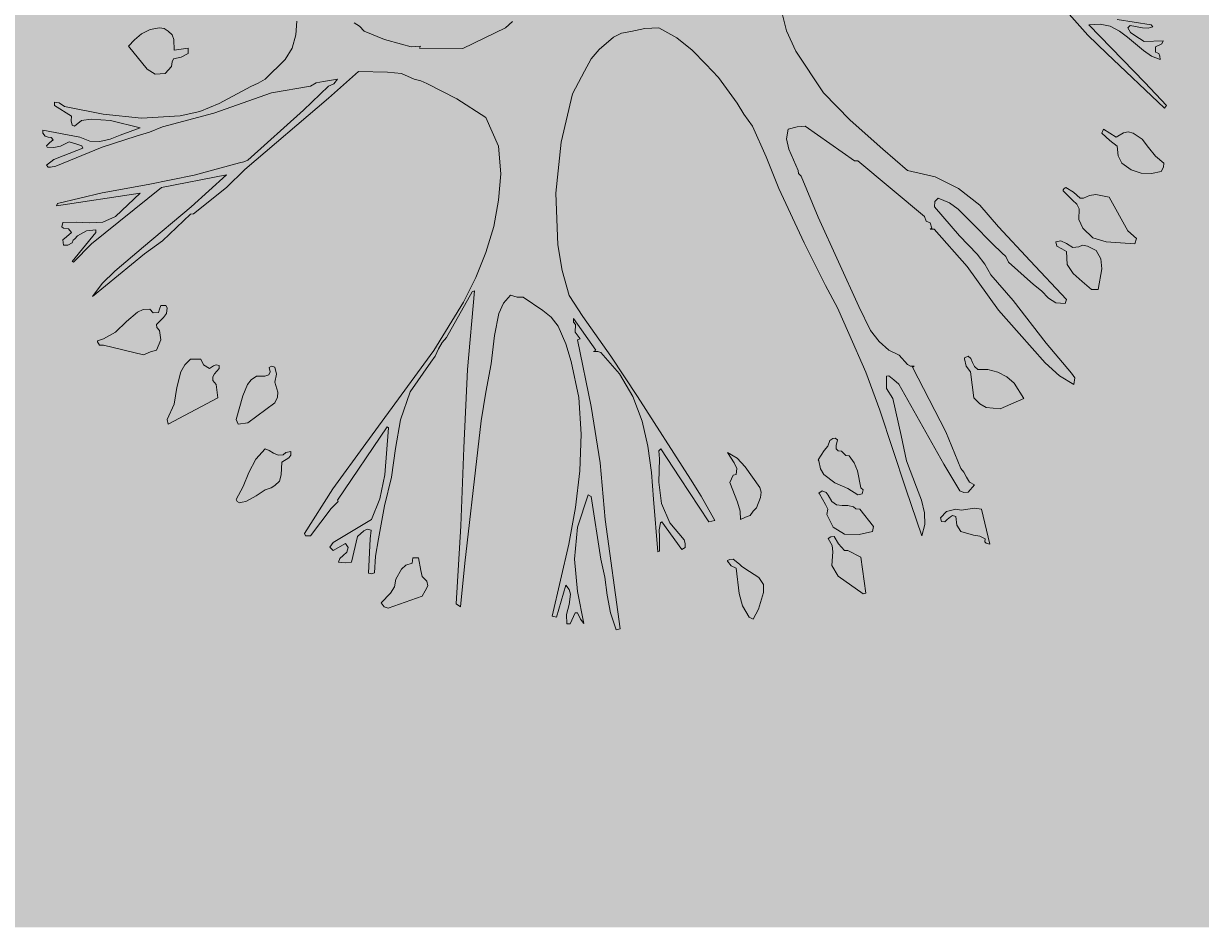
# Model space of a CAD drawing. Units: inches. Extents: x 84 to 1044, y -280 to 906.
# Tile 54 of 105: x 389 to 412, y 709 to 726. Entities that reach past the tile are written whole.
import ezdxf

# ---------------------------------------------------------------- set-up
doc = ezdxf.new("R2010")
doc.units = ezdxf.units.IN
doc.layers.add('A-ANNO-DIMS', color=2, linetype='Continuous', lineweight=18)
doc.layers.add('L-PLNT', color=114, linetype='Continuous', lineweight=15)
doc.layers.add('L-PLNT-PATT', color=9, linetype='Continuous', lineweight=9, true_color=0xafd9aa)
doc.styles.get("Standard").update_dxf_attribs({"font": 'arial.ttf'})
doc.dimstyles.get("Standard").update_dxf_attribs({"dimtxt": 0.18, "dimasz": 0.18, "dimexe": 0.18, "dimexo": 0.0625, "dimgap": 0.09, "dimtad": 0, "dimtih": 1, "dimtoh": 1, "dimdec": 4, "dimzin": 0, "dimdsep": 46, "dimtxsty": 'Standard', "dimcen": 0.09, "dimadec": 0, "dimazin": 0, "dimtfac": 1, "dimtdec": 4, "dimtofl": 0, "dimtmove": 0, "dimatfit": 3, "dimfxl": 1, "dimtolj": 1, "dimtzin": 0, "dimarcsym": 0})

# ---------------------------------------------------------------- blocks, each defined once
blk = doc.blocks.new('A$C37E508DF')
for p, q in [((0.9287, 0.7825), (0.936, 0.7542)), ((1.3151, 0.7487), (1.2919, 0.7752)), ((0.1244, 0.7504), (0.1351, 0.7559)), ((0.1351, 0.7559), (0.1471, 0.7577)), ((0.1471, 0.7577), (0.1527, 0.7568)), ((0.1527, 0.7568), (0.1578, 0.7538)), ((0.3186, 0.7491), (0.3199, 0.7662)), ((0.3919, 0.7641), (0.3988, 0.7598)), ((0.3988, 0.7598), (0.4043, 0.7538)), ((0.5287, 0.7319), (0.5823, 0.7577)), ((0.5823, 0.7577), (0.5913, 0.7658)), ((0.7577, 0.7568), (0.7401, 0.7534)), ((0.7752, 0.7577), (0.7577, 0.7568)), ((0.798, 0.7452), (0.7752, 0.7577)), ((1.3309, 0.7624), (1.3164, 0.7615)), ((1.3164, 0.7615), (1.3871, 0.6891)), ((1.3434, 0.7598), (1.3309, 0.7624)), ((1.355, 0.7538), (1.3434, 0.7598)), ((1.352, 0.7684), (1.3948, 0.7615)), ((1.3687, 0.7607), (1.3657, 0.7577)), ((1.3657, 0.7577), (1.3691, 0.7521)), ((1.3841, 0.7577), (1.3687, 0.7607)), ((1.3914, 0.7572), (1.3841, 0.7577)), ((1.397, 0.759), (1.3914, 0.7572)), ((1.3948, 0.7615), (1.397, 0.759)), ((0.1081, 0.7349), (0.1153, 0.7427)), ((0.1153, 0.7427), (0.1244, 0.7504)), ((0.1578, 0.7538), (0.1629, 0.7491)), ((0.1629, 0.7491), (0.1651, 0.7431)), ((0.1651, 0.7431), (0.1655, 0.7298)), ((0.3139, 0.7324), (0.3186, 0.7491)), ((0.4043, 0.7538), (0.4301, 0.7431)), ((0.4301, 0.7431), (0.4515, 0.7371)), ((0.7182, 0.7461), (0.7002, 0.7307)), ((0.7285, 0.7512), (0.7182, 0.7461)), ((0.7401, 0.7534), (0.7285, 0.7512)), ((0.8173, 0.7298), (0.798, 0.7452)), ((0.936, 0.7542), (0.9476, 0.7285)), ((1.3391, 0.7255), (1.3151, 0.7487)), ((1.3653, 0.7461), (1.355, 0.7538)), ((1.3854, 0.7294), (1.3653, 0.7461)), ((1.3691, 0.7521), (1.3743, 0.7482)), ((1.3743, 0.7482), (1.3863, 0.7405)), ((1.3863, 0.7405), (1.4099, 0.7414)), ((1.4099, 0.7414), (1.4086, 0.7375)), ((0.1312, 0.7058), (0.1081, 0.7349)), ((0.1655, 0.7298), (0.1831, 0.7324)), ((0.1831, 0.7324), (0.1831, 0.7255)), ((0.3049, 0.7178), (0.3139, 0.7324)), ((0.4515, 0.7371), (0.4635, 0.7341)), ((0.4635, 0.7341), (0.4755, 0.7349)), ((0.4755, 0.7349), (0.4742, 0.7324)), ((0.4742, 0.7324), (0.5287, 0.7319)), ((0.7002, 0.7307), (0.6903, 0.7186)), ((0.8344, 0.7122), (0.8173, 0.7298)), ((0.9476, 0.7285), (0.9828, 0.6762)), ((1.3953, 0.7221), (1.3854, 0.7294)), ((1.4086, 0.7375), (1.4004, 0.7337)), ((1.4004, 0.7337), (1.4004, 0.7272)), ((1.4004, 0.7272), (1.4047, 0.7255)), ((0.1629, 0.7152), (0.1621, 0.7092)), ((0.1646, 0.7186), (0.1629, 0.7152)), ((0.1741, 0.7208), (0.1646, 0.7186)), ((0.1831, 0.7255), (0.1741, 0.7208)), ((0.28, 0.6933), (0.3049, 0.7178)), ((0.6903, 0.7186), (0.6818, 0.7032)), ((0.8503, 0.6951), (0.8344, 0.7122)), ((1.4116, 0.6569), (1.3391, 0.7255)), ((1.4064, 0.7178), (1.3953, 0.7221)), ((1.4047, 0.7255), (1.406, 0.7221)), ((1.406, 0.7221), (1.4064, 0.7178)), ((0.1415, 0.6994), (0.1312, 0.7058)), ((0.1539, 0.7002), (0.1415, 0.6994)), ((0.1621, 0.7092), (0.1539, 0.7002)), ((0.3975, 0.7028), (0.3598, 0.6693)), ((0.4339, 0.7019), (0.3975, 0.7028)), ((0.4515, 0.7002), (0.4339, 0.7019)), ((0.4674, 0.6933), (0.4515, 0.7002)), ((0.6818, 0.7032), (0.6667, 0.6749)), ((0.2221, 0.6625), (0.262, 0.6839)), ((0.262, 0.6839), (0.271, 0.6882)), ((0.271, 0.6882), (0.28, 0.6933)), ((0.337, 0.6843), (0.2877, 0.6762)), ((0.328, 0.6543), (0.3598, 0.6843)), ((0.3443, 0.6886), (0.337, 0.6843)), ((0.3533, 0.6903), (0.3443, 0.6886)), ((0.3709, 0.6933), (0.3533, 0.6903)), ((0.3598, 0.6843), (0.3662, 0.6873)), ((0.3662, 0.6873), (0.3709, 0.6933)), ((0.476, 0.6912), (0.4674, 0.6933)), ((0.4832, 0.6878), (0.476, 0.6912)), ((0.521, 0.6685), (0.4832, 0.6878)), ((0.8739, 0.6629), (0.8503, 0.6951)), ((1.3871, 0.6891), (1.4141, 0.6599)), ((0.2877, 0.6762), (0.2152, 0.6505)), ((0.3598, 0.6693), (0.2543, 0.5797)), ((0.5578, 0.6449), (0.521, 0.6685)), ((0.6667, 0.6749), (0.6526, 0.614)), ((0.9828, 0.6762), (1.0162, 0.6415)), ((0.0146, 0.6599), (0.0146, 0.6642)), ((0.0146, 0.6642), (0.0206, 0.6633)), ((0.036, 0.6466), (0.0146, 0.6599)), ((0.0206, 0.6633), (0.0274, 0.6586)), ((0.0274, 0.6586), (0.0759, 0.6492)), ((0.1728, 0.647), (0.1977, 0.6526)), ((0.1977, 0.6526), (0.2221, 0.6625)), ((0.2581, 0.5913), (0.328, 0.6543)), ((0.8824, 0.6492), (0.8739, 0.6629)), ((1.4141, 0.6599), (1.4116, 0.6569)), ((0.0356, 0.6406), (0.036, 0.6466)), ((0.0369, 0.6355), (0.0356, 0.6406)), ((0.0489, 0.641), (0.0399, 0.6342)), ((0.0609, 0.6428), (0.0489, 0.641)), ((0.0853, 0.641), (0.0609, 0.6428)), ((0.0759, 0.6492), (0.1244, 0.644)), ((0.1226, 0.632), (0.0853, 0.641)), ((0.1244, 0.644), (0.1728, 0.647)), ((0.2152, 0.6505), (0.1509, 0.6333)), ((0.5737, 0.6089), (0.5578, 0.6449)), ((0.8932, 0.6342), (0.8824, 0.6492)), ((1.0162, 0.6415), (1.0574, 0.605)), ((0, 0.629), (0.0467, 0.62)), ((0, 0.6252), (0, 0.629)), ((0.003, 0.6213), (0, 0.6252)), ((0.0399, 0.6342), (0.0369, 0.6355)), ((0.0849, 0.6175), (0.0973, 0.6226)), ((0.0973, 0.6226), (0.1226, 0.632)), ((0.1342, 0.6265), (0.1175, 0.6213)), ((0.1509, 0.6333), (0.1342, 0.6265)), ((0.9103, 0.5956), (0.8932, 0.6342)), ((0.9382, 0.6303), (0.936, 0.6179)), ((0.9493, 0.6333), (0.9382, 0.6303)), ((0.9596, 0.6342), (0.9493, 0.6333)), ((1.0218, 0.5904), (0.9596, 0.6342)), ((1.3327, 0.6252), (1.3348, 0.6303)), ((1.343, 0.6162), (1.3327, 0.6252)), ((1.3348, 0.6303), (1.3511, 0.62)), ((1.3511, 0.62), (1.3601, 0.6256)), ((1.3601, 0.6256), (1.3661, 0.6269)), ((1.3661, 0.6269), (1.3725, 0.6252)), ((1.3725, 0.6252), (1.3837, 0.6175)), ((0.0069, 0.6204), (0.003, 0.6213)), ((0.0047, 0.6093), (0.0086, 0.6132)), ((0.0056, 0.6076), (0.0047, 0.6093)), ((0.0141, 0.6072), (0.0056, 0.6076)), ((0.0107, 0.6196), (0.0069, 0.6204)), ((0.0086, 0.6132), (0.0133, 0.617)), ((0.0133, 0.617), (0.0107, 0.6196)), ((0.0223, 0.6089), (0.0141, 0.6072)), ((0.0746, 0.6076), (0.0163, 0.5836)), ((0.0334, 0.6145), (0.0223, 0.6089)), ((0.0416, 0.6119), (0.0334, 0.6145)), ((0.0493, 0.6093), (0.0416, 0.6119)), ((0.0467, 0.62), (0.0592, 0.6153)), ((0.0506, 0.6063), (0.0493, 0.6093)), ((0.0592, 0.6153), (0.072, 0.6149)), ((0.072, 0.6149), (0.0849, 0.6175)), ((0.1175, 0.6213), (0.0746, 0.6076)), ((0.5763, 0.5741), (0.5737, 0.6089)), ((0.6526, 0.614), (0.6457, 0.5497)), ((0.936, 0.6179), (0.939, 0.605)), ((1.352, 0.6089), (1.343, 0.6162)), ((1.3533, 0.5969), (1.352, 0.6089)), ((1.3837, 0.6175), (1.3918, 0.6072)), ((0.0141, 0.5921), (0.0257, 0.5969)), ((0.0257, 0.5969), (0.0506, 0.6063)), ((0.9262, 0.5557), (0.9103, 0.5956)), ((0.939, 0.605), (0.9506, 0.5784)), ((1.0574, 0.605), (1.0883, 0.5784)), ((1.358, 0.5874), (1.3533, 0.5969)), ((1.3918, 0.6072), (1.4004, 0.5964)), ((1.4004, 0.5964), (1.4111, 0.5874)), ((0.0047, 0.5849), (0.0141, 0.5921)), ((0.0069, 0.5823), (0.0047, 0.5849)), ((0.0099, 0.5823), (0.0069, 0.5823)), ((0.0163, 0.5836), (0.0099, 0.5823)), ((0.1904, 0.5724), (0.2474, 0.5879)), ((0.2543, 0.5797), (0.2311, 0.557)), ((0.2474, 0.5879), (0.253, 0.5892)), ((0.253, 0.5892), (0.2581, 0.5913)), ((0.9506, 0.5784), (0.951, 0.5746)), ((1.0256, 0.5904), (1.0218, 0.5904)), ((1.1097, 0.5205), (1.0256, 0.5904)), ((1.0883, 0.5784), (1.123, 0.5703)), ((1.37, 0.5789), (1.358, 0.5874)), ((1.3824, 0.575), (1.37, 0.5789)), ((1.4103, 0.5823), (1.4077, 0.5771)), ((1.4111, 0.5874), (1.4103, 0.5823)), ((0.1325, 0.5608), (0.1904, 0.5724)), ((0.2311, 0.5729), (0.1496, 0.557)), ((0.1869, 0.5325), (0.2311, 0.5729)), ((0.5737, 0.5407), (0.5763, 0.5741)), ((0.951, 0.5746), (0.9545, 0.5711)), ((0.9545, 0.5711), (0.9759, 0.5193)), ((1.123, 0.5703), (1.1526, 0.5557)), ((1.3953, 0.5746), (1.3824, 0.575)), ((1.4077, 0.5771), (1.3953, 0.5746)), ((0.1226, 0.5497), (0.0171, 0.5338)), ((0.0184, 0.5368), (0.0746, 0.5501)), ((0.1496, 0.557), (0.0613, 0.4858)), ((0.0746, 0.5501), (0.1325, 0.5608)), ((0.0917, 0.5205), (0.1226, 0.5497)), ((0.2311, 0.557), (0.1899, 0.5235)), ((0.6457, 0.5497), (0.6483, 0.4845)), ((0.9583, 0.4871), (0.9262, 0.5557)), ((1.1526, 0.5557), (1.1792, 0.5347)), ((1.2842, 0.554), (1.2855, 0.5557)), ((1.2842, 0.5527), (1.2842, 0.554)), ((1.2958, 0.5407), (1.2842, 0.5527)), ((1.2855, 0.5557), (1.2876, 0.557)), ((1.2876, 0.557), (1.2971, 0.551)), ((1.2971, 0.551), (1.3057, 0.5433)), ((0.0171, 0.5338), (0.0184, 0.5368)), ((0.5677, 0.5077), (0.5737, 0.5407)), ((1.1226, 0.5394), (1.1221, 0.5325)), ((1.1268, 0.5433), (1.1226, 0.5394)), ((1.141, 0.5377), (1.1268, 0.5433)), ((1.1521, 0.5296), (1.141, 0.5377)), ((1.1792, 0.5347), (1.2027, 0.5072)), ((1.3014, 0.536), (1.2958, 0.5407)), ((1.3044, 0.53), (1.3014, 0.536)), ((1.3057, 0.5433), (1.3099, 0.5433)), ((1.3099, 0.5433), (1.3172, 0.5467)), ((1.3172, 0.5467), (1.3254, 0.548)), ((1.3254, 0.548), (1.3421, 0.5446)), ((1.3421, 0.5446), (1.3657, 0.5021)), ((0.0755, 0.5133), (0.0917, 0.5205)), ((0.1269, 0.482), (0.1869, 0.5325)), ((0.1861, 0.5231), (0.1509, 0.4897)), ((0.1899, 0.5235), (0.1861, 0.5231)), ((0.9759, 0.5193), (1.0269, 0.4069)), ((1.1118, 0.5145), (1.1097, 0.5205)), ((1.1221, 0.5325), (1.1539, 0.4961)), ((1.1706, 0.5111), (1.1521, 0.5296)), ((1.3039, 0.5167), (1.3044, 0.53)), ((0.024, 0.5072), (0.0253, 0.5128)), ((0.0262, 0.5055), (0.024, 0.5072)), ((0.0253, 0.5128), (0.042, 0.5133)), ((0.0326, 0.5047), (0.0262, 0.5055)), ((0.036, 0.5004), (0.0326, 0.5047)), ((0.042, 0.5133), (0.0587, 0.5124)), ((0.0587, 0.5124), (0.0755, 0.5133)), ((0.5578, 0.4751), (0.5677, 0.5077)), ((1.117, 0.5124), (1.1118, 0.5145)), ((1.1191, 0.5055), (1.117, 0.5124)), ((1.117, 0.5042), (1.1191, 0.5055)), ((1.1217, 0.5042), (1.117, 0.5042)), ((1.1633, 0.4575), (1.1217, 0.5042)), ((1.1955, 0.4858), (1.1706, 0.5111)), ((1.2027, 0.5072), (1.2426, 0.4644)), ((1.3091, 0.5055), (1.3039, 0.5167)), ((1.3215, 0.4935), (1.3091, 0.5055)), ((0.0253, 0.491), (0.03, 0.4948)), ((0.0262, 0.4841), (0.0253, 0.491)), ((0.03, 0.4948), (0.036, 0.5004)), ((0.0369, 0.4639), (0.0669, 0.5004)), ((0.0382, 0.4905), (0.0369, 0.4871)), ((0.0403, 0.4922), (0.0382, 0.4905)), ((0.0437, 0.4961), (0.0403, 0.4922)), ((0.0549, 0.5021), (0.0437, 0.4961)), ((0.0669, 0.5034), (0.0549, 0.5021)), ((0.0669, 0.5004), (0.0669, 0.5034)), ((0.1509, 0.4897), (0.1282, 0.4734)), ((1.1539, 0.4961), (1.1762, 0.4729)), ((1.2748, 0.4884), (1.2812, 0.4897)), ((1.2812, 0.4897), (1.2885, 0.4862)), ((1.3382, 0.4884), (1.3215, 0.4935)), ((1.3657, 0.5021), (1.3764, 0.4927)), ((1.3764, 0.4927), (1.3743, 0.4858)), ((0.0317, 0.4841), (0.0262, 0.4841)), ((0.0369, 0.4871), (0.0317, 0.4841)), ((0.0613, 0.4858), (0.0386, 0.4627)), ((0.0905, 0.4515), (0.1269, 0.482)), ((0.545, 0.4434), (0.5578, 0.4751)), ((0.6483, 0.4845), (0.6539, 0.4524)), ((0.9853, 0.4335), (0.9583, 0.4871)), ((1.207, 0.4747), (1.1955, 0.4858)), ((1.2122, 0.47), (1.207, 0.4747)), ((1.2761, 0.4832), (1.2748, 0.4884)), ((1.2825, 0.4798), (1.2761, 0.4832)), ((1.2885, 0.4764), (1.2825, 0.4798)), ((1.2885, 0.4862), (1.2962, 0.4815)), ((1.2894, 0.4601), (1.2885, 0.4764)), ((1.2962, 0.4815), (1.3039, 0.482)), ((1.3039, 0.482), (1.3087, 0.4841)), ((1.3087, 0.4841), (1.3147, 0.4832)), ((1.3147, 0.4832), (1.3258, 0.4777)), ((1.3258, 0.4777), (1.3318, 0.4669)), ((1.3743, 0.4858), (1.3382, 0.4884)), ((0.0386, 0.4627), (0.0369, 0.4639)), ((0.1282, 0.4734), (0.0626, 0.4198)), ((1.1762, 0.4729), (1.1856, 0.4605)), ((1.1856, 0.4605), (1.1933, 0.4468)), ((1.2156, 0.4627), (1.2122, 0.47)), ((1.2469, 0.4348), (1.2156, 0.4627)), ((1.2426, 0.4644), (1.2885, 0.4159)), ((1.2967, 0.4485), (1.2894, 0.4601)), ((1.3318, 0.4669), (1.3331, 0.4545)), ((0.0746, 0.4361), (0.0905, 0.4515)), ((0.6539, 0.4524), (0.6625, 0.4211)), ((1.2027, 0.4026), (1.1633, 0.4575)), ((1.1933, 0.4468), (1.2212, 0.4146)), ((1.3082, 0.4386), (1.2967, 0.4485)), ((1.3331, 0.4545), (1.3284, 0.4284)), ((0.0626, 0.4198), (0.0746, 0.4361)), ((0.5295, 0.4125), (0.545, 0.4434)), ((1.0003, 0.4052), (0.9853, 0.4335)), ((1.2568, 0.4266), (1.2469, 0.4348)), ((1.3198, 0.4284), (1.3082, 0.4386)), ((0.5403, 0.4254), (0.5081, 0.3679)), ((0.5347, 0.3276), (0.5433, 0.4266)), ((0.5433, 0.4266), (0.5403, 0.4254)), ((0.5887, 0.4215), (0.5797, 0.4112)), ((0.5969, 0.4189), (0.5887, 0.4215)), ((0.6046, 0.4189), (0.5969, 0.4189)), ((0.6295, 0.4022), (0.6046, 0.4189)), ((0.6625, 0.4211), (0.6796, 0.3945)), ((1.2658, 0.4176), (1.2568, 0.4266)), ((1.2752, 0.4116), (1.2658, 0.4176)), ((1.2885, 0.4159), (1.2868, 0.4108)), ((1.3284, 0.4284), (1.3198, 0.4284)), ((0.1055, 0.388), (0.1192, 0.4001)), ((0.1192, 0.4001), (0.1265, 0.4031)), ((0.1265, 0.4031), (0.1346, 0.4039)), ((0.1346, 0.4039), (0.1389, 0.3992)), ((0.1458, 0.3996), (0.1471, 0.4035)), ((0.1471, 0.4035), (0.1484, 0.4082)), ((0.1484, 0.4082), (0.1548, 0.4082)), ((0.1548, 0.4082), (0.1565, 0.4052)), ((0.1565, 0.4052), (0.1556, 0.3983)), ((0.4922, 0.3516), (0.5295, 0.4125)), ((0.5797, 0.4112), (0.5741, 0.3983)), ((0.6397, 0.3936), (0.6295, 0.4022)), ((1.0145, 0.373), (1.0003, 0.4052)), ((1.0269, 0.4069), (1.0419, 0.3769)), ((1.2289, 0.373), (1.2027, 0.4026)), ((1.2212, 0.4146), (1.2628, 0.361)), ((1.2868, 0.4108), (1.2752, 0.4116)), ((0.0917, 0.3748), (0.1055, 0.388)), ((0.1389, 0.3992), (0.1458, 0.3996)), ((0.1518, 0.3932), (0.1432, 0.3842)), ((0.1556, 0.3983), (0.1518, 0.3932)), ((0.5741, 0.3983), (0.5686, 0.3705)), ((0.6487, 0.3825), (0.6397, 0.3936)), ((0.6959, 0.352), (0.668, 0.3919)), ((0.668, 0.3919), (0.668, 0.3872)), ((0.668, 0.3872), (0.6706, 0.3842)), ((0.6796, 0.3945), (0.7148, 0.3447)), ((0.0763, 0.3662), (0.0917, 0.3748)), ((0.1432, 0.3842), (0.1436, 0.3808)), ((0.1436, 0.3808), (0.1471, 0.3769)), ((0.1471, 0.3769), (0.1484, 0.3649)), ((0.5686, 0.3705), (0.5643, 0.3349)), ((0.6582, 0.3602), (0.6487, 0.3825)), ((0.6706, 0.3842), (0.6702, 0.3748)), ((0.6702, 0.3748), (0.6762, 0.3662)), ((1.0359, 0.3246), (1.0145, 0.373)), ((1.0419, 0.3769), (1.0527, 0.3632)), ((1.2615, 0.3362), (1.2289, 0.373)), ((0.069, 0.364), (0.0763, 0.3662)), ((0.069, 0.3627), (0.069, 0.364)), ((0.0716, 0.3585), (0.069, 0.3627)), ((0.0763, 0.3585), (0.0716, 0.3585)), ((0.1269, 0.3464), (0.0763, 0.3585)), ((0.1484, 0.3649), (0.1432, 0.352)), ((0.5025, 0.3619), (0.4982, 0.3537)), ((0.5081, 0.3679), (0.5025, 0.3619)), ((0.665, 0.3379), (0.6582, 0.3602)), ((0.6762, 0.3662), (0.6732, 0.3653)), ((0.6732, 0.3653), (0.6903, 0.2813)), ((1.0527, 0.3632), (1.0647, 0.352)), ((1.2628, 0.361), (1.2949, 0.3233)), ((0.1355, 0.3499), (0.1269, 0.3464)), ((0.1432, 0.352), (0.1355, 0.3499)), ((0.1788, 0.3336), (0.1861, 0.3409)), ((0.1861, 0.3409), (0.199, 0.3409)), ((0.199, 0.3409), (0.2024, 0.3336)), ((0.4065, 0.2345), (0.4922, 0.3516)), ((0.4939, 0.3447), (0.4884, 0.337)), ((0.4982, 0.3537), (0.4939, 0.3447)), ((0.6933, 0.3503), (0.6959, 0.352)), ((0.6985, 0.3503), (0.6933, 0.3503)), ((0.7023, 0.349), (0.6985, 0.3503)), ((0.7259, 0.3224), (0.7023, 0.349)), ((0.7148, 0.3447), (0.7487, 0.2937)), ((1.0647, 0.352), (1.078, 0.346)), ((1.078, 0.346), (1.0883, 0.334)), ((1.1599, 0.3426), (1.1646, 0.3447)), ((1.1599, 0.3413), (1.1599, 0.3426)), ((1.162, 0.3319), (1.1599, 0.3413)), ((1.1646, 0.3447), (1.168, 0.3417)), ((1.168, 0.3417), (1.1702, 0.3366)), ((0.1737, 0.325), (0.1788, 0.3336)), ((0.2024, 0.3336), (0.2097, 0.3289)), ((0.2097, 0.3289), (0.2148, 0.3323)), ((0.2148, 0.3323), (0.2182, 0.3336)), ((0.2221, 0.3289), (0.2161, 0.3224)), ((0.2182, 0.3336), (0.2221, 0.3327)), ((0.2221, 0.3327), (0.2221, 0.3289)), ((0.2851, 0.3302), (0.2877, 0.3319)), ((0.2864, 0.325), (0.2851, 0.3302)), ((0.2877, 0.3319), (0.292, 0.3306)), ((0.292, 0.3306), (0.2941, 0.322)), ((0.4884, 0.337), (0.4622, 0.2997)), ((0.53, 0.229), (0.5347, 0.3276)), ((0.5643, 0.3349), (0.5578, 0.2993)), ((0.6745, 0.2924), (0.665, 0.3379)), ((1.0883, 0.334), (1.0921, 0.3319)), ((1.0921, 0.3319), (1.0968, 0.3319)), ((1.0968, 0.3319), (1.0947, 0.3306)), ((1.0947, 0.3306), (1.1367, 0.2491)), ((1.1676, 0.325), (1.162, 0.3319)), ((1.1702, 0.3366), (1.1727, 0.3314)), ((1.1727, 0.3314), (1.177, 0.3276)), ((1.177, 0.3276), (1.1895, 0.3276)), ((1.1895, 0.3276), (1.2019, 0.3246)), ((1.2795, 0.3199), (1.2615, 0.3362)), ((0.1689, 0.3053), (0.1737, 0.325)), ((0.2161, 0.3224), (0.214, 0.3186)), ((0.214, 0.3186), (0.214, 0.3139)), ((0.214, 0.3139), (0.2182, 0.3087)), ((0.2577, 0.3087), (0.2624, 0.3147)), ((0.2624, 0.3147), (0.2689, 0.3194)), ((0.2689, 0.3194), (0.2796, 0.3194)), ((0.2796, 0.3194), (0.2847, 0.3211)), ((0.2847, 0.3211), (0.2864, 0.325)), ((0.2941, 0.322), (0.292, 0.3117)), ((0.292, 0.3117), (0.2959, 0.2993)), ((0.7427, 0.2937), (0.7259, 0.3224)), ((1.0535, 0.2766), (1.0359, 0.3246)), ((1.0647, 0.3199), (1.0617, 0.3194)), ((1.0617, 0.3194), (1.0617, 0.304)), ((1.0711, 0.3147), (1.0647, 0.3199)), ((1.0775, 0.3092), (1.0711, 0.3147)), ((1.1719, 0.292), (1.1676, 0.325)), ((1.2019, 0.3246), (1.2135, 0.3186)), ((1.2135, 0.3186), (1.2225, 0.3104)), ((1.2975, 0.3087), (1.2795, 0.3199)), ((1.2949, 0.3233), (1.2988, 0.3173)), ((1.2988, 0.3173), (1.2975, 0.3087)), ((0.1655, 0.2843), (0.1689, 0.3053)), ((0.2182, 0.3087), (0.2204, 0.292)), ((0.2517, 0.2946), (0.2577, 0.3087)), ((0.2959, 0.2993), (0.2954, 0.2928)), ((0.4622, 0.2997), (0.4502, 0.2645)), ((0.5578, 0.2993), (0.5518, 0.2633)), ((1.0617, 0.304), (1.0698, 0.2911)), ((1.1341, 0.2084), (1.0775, 0.3092)), ((1.2225, 0.3104), (1.2349, 0.2911)), ((0.1565, 0.265), (0.1655, 0.2843)), ((0.2204, 0.292), (0.1578, 0.259)), ((0.2436, 0.265), (0.2517, 0.2946)), ((0.292, 0.286), (0.2581, 0.2607)), ((0.2954, 0.2928), (0.292, 0.286)), ((0.6775, 0.2465), (0.6745, 0.2924)), ((0.7542, 0.2628), (0.7427, 0.2937)), ((0.7487, 0.2937), (0.8151, 0.1899)), ((1.0698, 0.2911), (1.0805, 0.2448)), ((1.1792, 0.2847), (1.1719, 0.292)), ((1.1873, 0.28), (1.1792, 0.2847)), ((1.2349, 0.2911), (1.2049, 0.2783)), ((0.6903, 0.2813), (0.7015, 0.2101)), ((1.0861, 0.1775), (1.0535, 0.2766)), ((1.2049, 0.2783), (1.1873, 0.28)), ((0.1578, 0.259), (0.1565, 0.265)), ((0.2461, 0.259), (0.2436, 0.265)), ((0.2581, 0.2607), (0.2461, 0.259)), ((0.4335, 0.2556), (0.3709, 0.1634)), ((0.4305, 0.1951), (0.4352, 0.2543)), ((0.4352, 0.2543), (0.4335, 0.2556)), ((0.4502, 0.2645), (0.4438, 0.2285)), ((0.5518, 0.2633), (0.5475, 0.2268)), ((0.7615, 0.2311), (0.7542, 0.2628)), ((0.6758, 0.2002), (0.6775, 0.2465)), ((0.9879, 0.2311), (0.9905, 0.2384)), ((0.9905, 0.2384), (0.9943, 0.241)), ((0.9943, 0.241), (0.9973, 0.2414)), ((0.9973, 0.2414), (1.0003, 0.2393)), ((1.0003, 0.2393), (0.9986, 0.232)), ((1.0805, 0.2448), (1.087, 0.2127)), ((1.1367, 0.2491), (1.1556, 0.2032)), ((0.268, 0.2148), (0.28, 0.2277)), ((0.28, 0.2277), (0.2851, 0.226)), ((0.2851, 0.226), (0.2903, 0.2225)), ((0.2903, 0.2225), (0.2963, 0.22)), ((0.3027, 0.2204), (0.3061, 0.2234)), ((0.3061, 0.2234), (0.3122, 0.2247)), ((0.3122, 0.2247), (0.3122, 0.22)), ((0.3649, 0.1775), (0.4065, 0.2345)), ((0.4438, 0.2285), (0.4391, 0.1921)), ((0.5261, 0.1308), (0.53, 0.229)), ((0.5475, 0.2268), (0.5313, 0.084)), ((0.7662, 0.1981), (0.7615, 0.2311)), ((0.7778, 0.2277), (0.7752, 0.2255)), ((0.7752, 0.2255), (0.7761, 0.2152)), ((0.8018, 0.1912), (0.7778, 0.2277)), ((0.8619, 0.2234), (0.8739, 0.2161)), ((0.87, 0.2101), (0.8619, 0.2234)), ((0.9759, 0.214), (0.9836, 0.226)), ((0.9836, 0.226), (0.9879, 0.2311)), ((0.9986, 0.232), (0.9986, 0.2281)), ((0.9986, 0.2281), (1.0012, 0.2255)), ((1.0012, 0.2255), (1.0051, 0.2251)), ((1.0051, 0.2251), (1.0076, 0.2225)), ((1.0076, 0.2225), (1.0106, 0.2195)), ((0.2594, 0.1981), (0.268, 0.2148)), ((0.2963, 0.22), (0.3027, 0.2204)), ((0.301, 0.211), (0.3002, 0.1951)), ((0.3096, 0.2165), (0.301, 0.211)), ((0.3122, 0.22), (0.3096, 0.2165)), ((0.7015, 0.2101), (0.7079, 0.1389)), ((0.7761, 0.2152), (0.7752, 0.1861)), ((0.8734, 0.2032), (0.87, 0.2101)), ((0.8739, 0.2161), (0.8841, 0.2054)), ((0.9768, 0.2127), (0.9759, 0.214)), ((0.9789, 0.2028), (0.9768, 0.2127)), ((1.0106, 0.2195), (1.0149, 0.2191)), ((1.0149, 0.2191), (1.0214, 0.2101)), ((1.0214, 0.2101), (1.0252, 0.2002)), ((1.087, 0.2127), (1.0998, 0.1797)), ((1.1543, 0.1749), (1.1341, 0.2084)), ((0.2521, 0.1805), (0.2594, 0.1981)), ((0.3002, 0.1951), (0.298, 0.1874)), ((0.4241, 0.1651), (0.4305, 0.1951)), ((0.6706, 0.1539), (0.6758, 0.2002)), ((0.7688, 0.1646), (0.7662, 0.1981)), ((0.8649, 0.1857), (0.8687, 0.1947)), ((0.8687, 0.1947), (0.8726, 0.1955)), ((0.8726, 0.1955), (0.8734, 0.2032)), ((0.8841, 0.2054), (0.9026, 0.1792)), ((0.9832, 0.1955), (0.9789, 0.2028)), ((0.9969, 0.1852), (0.9832, 0.1955)), ((1.0252, 0.2002), (1.0295, 0.1788)), ((1.1556, 0.2032), (1.1594, 0.1985)), ((1.1594, 0.1985), (1.1624, 0.1921)), ((0.2436, 0.1642), (0.2521, 0.1805)), ((0.2873, 0.1788), (0.28, 0.1762)), ((0.292, 0.1818), (0.2873, 0.1788)), ((0.298, 0.1874), (0.292, 0.1818)), ((0.4391, 0.1921), (0.4301, 0.1561)), ((0.7752, 0.1861), (0.7787, 0.1591)), ((0.8383, 0.1359), (0.8018, 0.1912)), ((0.8151, 0.1899), (0.8288, 0.1685)), ((0.8743, 0.1608), (0.8649, 0.1857)), ((0.9026, 0.1792), (0.9043, 0.1732)), ((1.0132, 0.1779), (0.9969, 0.1852)), ((1.0256, 0.1698), (1.0132, 0.1779)), ((1.0295, 0.1788), (1.0325, 0.1762)), ((1.0998, 0.1797), (1.1058, 0.1634)), ((1.1624, 0.1921), (1.1663, 0.1861)), ((1.1727, 0.1827), (1.1646, 0.1732)), ((1.1663, 0.1861), (1.1727, 0.1827)), ((0.2448, 0.1616), (0.2436, 0.1642)), ((0.2684, 0.1689), (0.2556, 0.1616)), ((0.28, 0.1762), (0.2684, 0.1689)), ((0.3293, 0.1213), (0.3649, 0.1775)), ((0.3709, 0.1634), (0.3718, 0.1616)), ((0.4138, 0.1389), (0.4241, 0.1651)), ((0.6865, 0.1698), (0.6732, 0.1295)), ((0.6903, 0.1681), (0.6865, 0.1698)), ((0.7023, 0.0892), (0.6903, 0.1681)), ((0.774, 0.0982), (0.7688, 0.1646)), ((0.8288, 0.1685), (0.846, 0.1376)), ((0.9035, 0.1668), (0.8983, 0.1535)), ((0.9043, 0.1732), (0.9035, 0.1668)), ((0.9768, 0.1719), (0.9811, 0.1749)), ((0.9776, 0.1711), (0.9768, 0.1719)), ((0.9853, 0.1578), (0.9776, 0.1711)), ((0.9811, 0.1749), (0.9858, 0.1728)), ((0.9858, 0.1728), (0.9884, 0.1694)), ((0.9884, 0.1694), (0.9931, 0.1616)), ((1.0312, 0.1711), (1.0256, 0.1698)), ((1.0325, 0.1762), (1.0312, 0.1711)), ((1.1063, 0.1183), (1.0861, 0.1775)), ((1.1058, 0.1634), (1.1097, 0.1475)), ((1.1594, 0.1728), (1.1543, 0.1749)), ((1.1646, 0.1732), (1.1594, 0.1728)), ((0.2478, 0.1599), (0.2448, 0.1616)), ((0.2508, 0.1608), (0.2478, 0.1599)), ((0.2556, 0.1616), (0.2508, 0.1608)), ((0.3628, 0.1526), (0.337, 0.1183)), ((0.3692, 0.1591), (0.3628, 0.1526)), ((0.3718, 0.1616), (0.3692, 0.1591)), ((0.4301, 0.1561), (0.4224, 0.1145)), ((0.662, 0.108), (0.6706, 0.1539)), ((0.7787, 0.1591), (0.789, 0.1346)), ((0.8777, 0.1496), (0.8743, 0.1608)), ((0.8781, 0.1389), (0.8777, 0.1496)), ((0.894, 0.1496), (0.8902, 0.1441)), ((0.8983, 0.1535), (0.894, 0.1496)), ((0.9879, 0.1518), (0.9853, 0.1578)), ((0.9866, 0.1453), (0.9879, 0.1518)), ((0.9931, 0.1616), (0.9991, 0.1574)), ((0.9991, 0.1574), (1.0059, 0.1565)), ((1.0059, 0.1565), (1.0132, 0.1565)), ((1.0132, 0.1565), (1.0205, 0.1548)), ((1.0205, 0.1548), (1.0235, 0.1522)), ((1.0235, 0.1522), (1.0282, 0.1518)), ((1.0282, 0.1518), (1.0454, 0.1303)), ((1.1298, 0.1411), (1.1376, 0.1492)), ((1.1376, 0.1492), (1.1491, 0.1518)), ((1.1491, 0.1518), (1.1564, 0.1505)), ((1.1564, 0.1505), (1.1642, 0.1518)), ((1.1642, 0.1518), (1.1727, 0.1531)), ((1.1727, 0.1531), (1.1813, 0.1518)), ((1.1813, 0.1518), (1.192, 0.108)), ((0.3653, 0.1098), (0.4138, 0.1389)), ((0.7079, 0.1389), (0.7268, 0.0013)), ((0.7774, 0.1346), (0.7757, 0.1261)), ((0.7791, 0.1359), (0.7774, 0.1346)), ((0.8044, 0.1012), (0.7791, 0.1359)), ((0.789, 0.1346), (0.8074, 0.1132)), ((0.846, 0.1376), (0.8383, 0.1359)), ((0.8846, 0.1419), (0.8781, 0.1389)), ((0.8902, 0.1441), (0.8846, 0.1419)), ((0.9948, 0.1291), (0.9866, 0.1453)), ((1.1097, 0.1475), (1.1101, 0.1325)), ((1.1311, 0.1364), (1.1298, 0.1411)), ((1.1354, 0.1359), (1.1311, 0.1364)), ((1.1384, 0.1389), (1.1354, 0.1359)), ((1.1423, 0.1423), (1.1384, 0.1389)), ((1.1449, 0.1441), (1.1423, 0.1423)), ((1.1491, 0.1428), (1.1449, 0.1441)), ((1.1504, 0.132), (1.1491, 0.1428)), ((0.3306, 0.1183), (0.3293, 0.1213)), ((0.4039, 0.1248), (0.3962, 0.1175)), ((0.4082, 0.1269), (0.4039, 0.1248)), ((0.4134, 0.1256), (0.4082, 0.1269)), ((0.4121, 0.1145), (0.4134, 0.1256)), ((0.5205, 0.033), (0.5261, 0.1308)), ((0.6732, 0.1295), (0.6693, 0.0892)), ((0.7757, 0.1261), (0.7761, 0.117)), ((1.0089, 0.1205), (0.9948, 0.1291)), ((1.0274, 0.12), (1.0089, 0.1205)), ((1.0441, 0.1239), (1.0274, 0.12)), ((1.0454, 0.1303), (1.0441, 0.1239)), ((1.1101, 0.1325), (1.1063, 0.1183)), ((1.1556, 0.1239), (1.1504, 0.132)), ((1.1714, 0.1192), (1.1556, 0.1239)), ((1.1792, 0.1179), (1.1714, 0.1192)), ((0.337, 0.1183), (0.3306, 0.1183)), ((0.3615, 0.1042), (0.3653, 0.1098)), ((0.3653, 0.0999), (0.3615, 0.1042)), ((0.3812, 0.1089), (0.3653, 0.0999)), ((0.3842, 0.1037), (0.3812, 0.1089)), ((0.3825, 0.0978), (0.3842, 0.1037)), ((0.3962, 0.1175), (0.3885, 0.0853)), ((0.4099, 0.0716), (0.4121, 0.1145)), ((0.4224, 0.1145), (0.4189, 0.093)), ((0.641, 0.0172), (0.662, 0.108)), ((0.7761, 0.117), (0.7761, 0.099)), ((0.8083, 0.1037), (0.8044, 0.1012)), ((0.8074, 0.1132), (0.8087, 0.1089)), ((0.8087, 0.1089), (0.8083, 0.1037)), ((0.9884, 0.1149), (0.9918, 0.117)), ((0.9935, 0.1063), (0.9884, 0.1149)), ((0.9918, 0.117), (0.9961, 0.1175)), ((0.9943, 0.0982), (0.9935, 0.1063)), ((0.9961, 0.1175), (1.0016, 0.1085)), ((1.0016, 0.1085), (1.0089, 0.0999)), ((1.186, 0.1145), (1.1792, 0.1179)), ((1.1856, 0.111), (1.186, 0.1145)), ((1.1873, 0.1093), (1.1856, 0.111)), ((1.192, 0.108), (1.1873, 0.1093)), ((0.3722, 0.0853), (0.3739, 0.09)), ((0.3739, 0.09), (0.3782, 0.0935)), ((0.3782, 0.0935), (0.3825, 0.0978)), ((0.4189, 0.093), (0.4176, 0.072)), ((0.4648, 0.084), (0.4657, 0.0905)), ((0.4657, 0.0905), (0.473, 0.0905)), ((0.473, 0.0905), (0.476, 0.0746)), ((0.6693, 0.0892), (0.6728, 0.0484)), ((0.7075, 0.0665), (0.7023, 0.0892)), ((0.7761, 0.099), (0.774, 0.0982)), ((0.8649, 0.0887), (0.8691, 0.0892)), ((0.8691, 0.0892), (0.8769, 0.0827)), ((0.9931, 0.081), (0.9943, 0.0982)), ((1.0089, 0.0999), (1.0132, 0.0999)), ((1.0132, 0.0999), (1.0295, 0.0917)), ((1.0295, 0.0917), (1.0359, 0.0463)), ((0.3808, 0.0845), (0.3722, 0.0853)), ((0.3885, 0.0853), (0.3808, 0.0845)), ((0.4442, 0.0639), (0.4515, 0.0763)), ((0.4515, 0.0763), (0.4571, 0.0815)), ((0.4571, 0.0815), (0.4648, 0.084)), ((0.476, 0.0746), (0.4777, 0.0673)), ((0.5313, 0.084), (0.5257, 0.0291)), ((0.8619, 0.0875), (0.8649, 0.0887)), ((0.8619, 0.0866), (0.8619, 0.0875)), ((0.8666, 0.0806), (0.8619, 0.0866)), ((0.8726, 0.0776), (0.8666, 0.0806)), ((0.8764, 0.0459), (0.8726, 0.0776)), ((0.8769, 0.0827), (0.8799, 0.0797)), ((0.8799, 0.0797), (0.8893, 0.0733)), ((1.0012, 0.0677), (0.9931, 0.081)), ((0.4142, 0.0707), (0.4099, 0.0716)), ((0.4176, 0.072), (0.4142, 0.0707)), ((0.4425, 0.0544), (0.4442, 0.0639)), ((0.4777, 0.0673), (0.4832, 0.0613)), ((0.4832, 0.0613), (0.4845, 0.0553)), ((0.7105, 0.0437), (0.7075, 0.0665)), ((0.8893, 0.0733), (0.9013, 0.066)), ((0.9013, 0.066), (0.9069, 0.057)), ((1.0325, 0.0454), (1.0012, 0.0677)), ((0.4258, 0.0339), (0.4378, 0.0463)), ((0.4378, 0.0463), (0.4425, 0.0544)), ((0.4811, 0.0493), (0.4777, 0.0424)), ((0.4845, 0.0553), (0.4811, 0.0493)), ((0.6582, 0.0562), (0.6466, 0.0159)), ((0.6625, 0.051), (0.6582, 0.0562)), ((0.6642, 0.045), (0.6625, 0.051)), ((0.6625, 0.0321), (0.6642, 0.045)), ((0.6728, 0.0484), (0.6809, 0.0082)), ((0.8807, 0.0304), (0.8764, 0.0459)), ((0.9069, 0.0471), (0.9009, 0.0261)), ((0.9069, 0.057), (0.9069, 0.0471)), ((1.0359, 0.0463), (1.0325, 0.0454)), ((0.4296, 0.0291), (0.4258, 0.0339)), ((0.4777, 0.0424), (0.4348, 0.0274)), ((0.5257, 0.0291), (0.5205, 0.033)), ((0.659, 0.0193), (0.6625, 0.0321)), ((0.7144, 0.0214), (0.7105, 0.0437)), ((0.8889, 0.0159), (0.8807, 0.0304)), ((0.4348, 0.0274), (0.4296, 0.0291)), ((0.6466, 0.0159), (0.641, 0.0172)), ((0.6595, 0.0077), (0.659, 0.0193)), ((0.6702, 0.0214), (0.6637, 0.0077)), ((0.6732, 0.0214), (0.6702, 0.0214)), ((0.6766, 0.0133), (0.6732, 0.0214)), ((0.7216, 0), (0.7144, 0.0214)), ((0.894, 0.0137), (0.8889, 0.0159)), ((0.9009, 0.0261), (0.894, 0.0137)), ((0.6637, 0.0077), (0.6595, 0.0077)), ((0.6809, 0.0082), (0.6766, 0.0133)), ((0.7268, 0.0013), (0.7216, 0))]:
    blk.add_line(p, q)
blk = doc.blocks.new('*D62')
at = {"layer": 'A-ANNO-DIMS', "color": 0, "lineweight": -2, "transparency": 16777216}
for p, q in [((203.179, 709.183), (203.179, 905.9)), ((896.074, 400.183), (896.074, 905.9)), ((203.359, 905.72), (549.232, 905.72)), ((895.894, 905.72), (550.021, 905.72))]:
    blk.add_line(p, q, dxfattribs=at)
at = {"layer": 'A-ANNO-DIMS', "color": 0, "transparency": 16777216}
for points in [[(203.359, 905.75), (203.359, 905.69), (203.179, 905.72)], [(895.894, 905.75), (895.894, 905.69), (896.074, 905.72)]]:
    blk.add_solid(points, dxfattribs=at)
at = {"layer": 'Defpoints', "color": 0, "transparency": 16777216}
for p in [(896.074, 905.72), (203.179, 709.12), (896.074, 400.12)]:
    blk.add_point(p, dxfattribs=at)
at = {"layer": 'A-ANNO-DIMS', "color": 0, "transparency": 16777216, "insert": (549.627, 905.72), "char_height": 0.18, "attachment_point": 5}
blk.add_mtext('\\A1;692.9', dxfattribs=at)

msp = doc.modelspace()

# ---------------------------------------------------------------- hatches: boundary and pattern name
at = {"layer": 'L-PLNT-PATT', "transparency": 33554597}
h = msp.add_hatch(color=256, dxfattribs=at)
h.dxf.hatch_style = 1
h.paths.add_polyline_path([(434.074, 769.12), (386.074, 769.12), (386.074, 709.12), (434.074, 709.12)])
h.paths.add_polyline_path([(896.074, 847.12), (434.074, 847.12), (434.074, 769.12), (434.074, 709.12), (470.074, 709.12), (506.074, 709.12), (572.074, 709.12), (608.074, 709.12), (698.074, 709.12), (770.074, 709.12), (833.074, 709.12), (896.074, 709.12)])
h.paths.add_polyline_path([(983.074, 847.12), (896.074, 847.12), (896.074, 709.12), (896.074, 547.12), (932.074, 547.12), (983.074, 547.12)])
h.paths.add_polyline_path([(983.074, 547.12), (932.074, 547.12), (932.074, 265.12), (983.074, 265.12)])
h.paths.add_polyline_path([(203.179, 646.12), (203.179, 709.12), (203.179, 745.12), (143.179, 745.12), (143.179, 271.12), (203.179, 271.12), (203.179, 274.12), (203.179, 310.12), (203.179, 574.12)])

# ---------------------------------------------------------------- block references
at = {"layer": 'L-PLNT', "xscale": 15.19586232982809, "yscale": 15.19586232982809, "zscale": 15.19586232982809}
msp.add_blockref('A$C37E508DF', (389.477, 714.812), dxfattribs=at)

# ---------------------------------------------------------------- dimensions: what is measured, and where the dimension line sits
at = {"layer": 'A-ANNO-DIMS'}
dim = msp.add_linear_dim(base=(896.074, 905.72), p1=(203.179, 709.12), p2=(896.074, 400.12), dimstyle='Standard', override={"dimdec": 1, "dimlfac": 1, "dimrnd": 0, "dimzin": 0, "dimdsep": 46, "dimlunit": 2}, dxfattribs=at)
dim.commit()
dim.dimension.update_dxf_attribs({"geometry": '*D62', "text_midpoint": (549.627, 905.72)})

doc.saveas('drawing.dxf')
